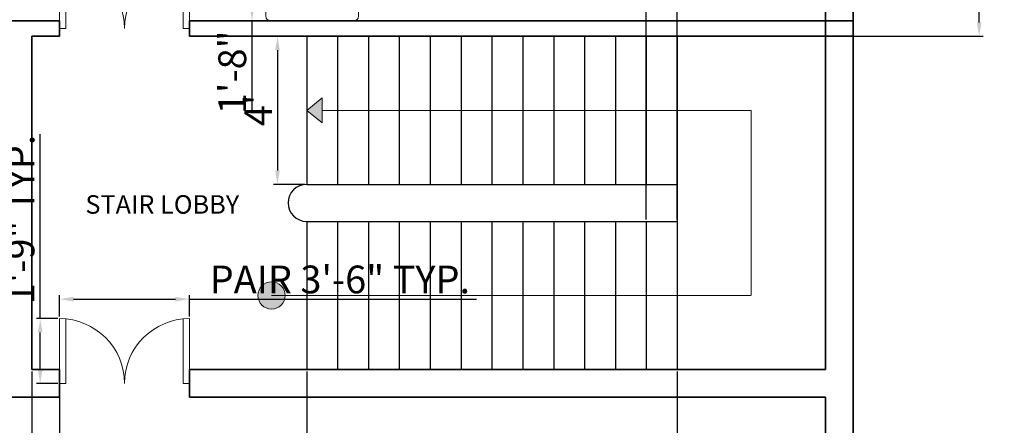
# Model space of a CAD drawing. Units: inches. Extents: x 1885 to 4781, y 1153 to 4395.
# Tile 4 of 7: x 2631 to 2950, y 1657 to 1789. Entities that reach past the tile are written whole.
import ezdxf

# ---------------------------------------------------------------- set-up
doc = ezdxf.new("R2010")
doc.units = ezdxf.units.IN
for name, color, linetype, lineweight in [('A-ANNO-DIMS', 5, 'Continuous', 18), ('A-ANNO-SYMB', 7, 'Continuous', 18), ('A-FLOR-STRS', 7, 'Continuous', 25), ('A-WALL', 7, 'Continuous', 35)]:
    doc.layers.add(name, color=color, linetype=linetype, lineweight=lineweight)
for name, color, linetype, lineweight, true_color in [('A-AREA-IDEN', 244, 'Continuous', 18, 0x991b1e), ('A-DOOR', 11, 'Continuous', 18, 0xf27172), ('A-FLOR-FIXT', 11, 'Continuous', 18, 0xf27172)]:
    doc.layers.add(name, color=color, linetype=linetype, lineweight=lineweight, true_color=true_color)
doc.styles.get("Standard").update_dxf_attribs({"font": 'arial.ttf'})
doc.dimstyles.new('ISO-25', dxfattribs={"dimtxt": 9, "dimasz": 4.5, "dimexe": 1.25, "dimexo": 0.625, "dimtad": 1, "dimdec": 0, "dimlunit": 3, "dimtxsty": 'Standard', "dimcen": 2.5, "dimadec": 0, "dimazin": 0, "dimtfac": 1, "dimtdec": 0, "dimtmove": 0, "dimatfit": 3, "dimfxl": 1, "dimarcsym": 0})

# ---------------------------------------------------------------- blocks, each defined once
blk = doc.blocks.new('Sink-single - 30 in top')
blk.add_line((-15, -3.999996), (15, -3.999996))
for points in [[(-13.5, 0), (13.5, 0)], [(-15, -18.499996), (-15, -1.5)], [(15, -1.5), (15, -18.499996)], [(-12.5, -5.499996), (12.5, -5.499996)], [(-13.5, -17.499996), (-13.5, -6.499996)], [(13.5, -6.499996), (13.5, -17.499996)], [(12.5, -18.499996), (-12.5, -18.499996)], [(13.5, -19.999996), (-13.5, -19.999996)]]:
    blk.add_lwpolyline(points)
for radius in [1, 0.5]:
    blk.add_circle((0, -11.999996), radius)
for centre, radius, start, end in [((-13.5, -1.5), 1.5, 90, 180), ((13.5, -1.5), 1.5, 0, 90), ((-12.5, -6.499996), 1, 90, 180), ((12.5, -6.499996), 1, 0, 90), ((-13.5, -18.499996), 1.5, 180, 270), ((-12.5, -17.499996), 1, 180, 270), ((12.5, -17.499996), 1, 270, 0), ((13.5, -18.499996), 1.5, 270, 0)]:
    blk.add_arc(centre, radius, start, end)
blk = doc.blocks.new('*D22')
at = {"layer": 'A-ANNO-DIMS', "color": 0, "lineweight": -2, "transparency": 16777216}
for p, q in [((2723.28, 1783.42), (2713.21, 1783.42)), ((2714.46, 1778.92), (2714.46, 1739.92)), ((2723.28, 1735.42), (2713.21, 1735.42))]:
    blk.add_line(p, q, dxfattribs=at)
at = {"layer": 'A-ANNO-DIMS', "color": 0, "transparency": 16777216}
for points in [[(2713.71, 1778.92), (2715.21, 1778.92), (2714.46, 1783.42)], [(2713.71, 1739.92), (2715.21, 1739.92), (2714.46, 1735.42)]]:
    blk.add_solid(points, dxfattribs=at)
at = {"layer": 'Defpoints', "color": 0, "transparency": 16777216}
for p in [(2723.91, 1783.42), (2714.46, 1735.42), (2723.91, 1735.42)]:
    blk.add_point(p, dxfattribs=at)
at = {"layer": 'A-ANNO-DIMS', "color": 0, "transparency": 16777216, "insert": (2709.34, 1759.42), "char_height": 9, "attachment_point": 5, "rotation": 90}
blk.add_mtext("4'", dxfattribs=at)
blk = doc.blocks.new('DOOR-PAIR-42IN')
for p, q in [((0, 21), (0, 0)), ((2, 21), (2, 0)), ((40, 21), (40, 0)), ((42, 21), (42, 0)), ((0, 0), (2, 0)), ((42, 0), (40, 0))]:
    blk.add_line(p, q)
for centre, start, end in [((0, 0), 0, 90), ((42, 0), 90, 180)]:
    blk.add_arc(centre, 21, start, end)
blk = doc.blocks.new('*D55')
at = {"layer": 'A-ANNO-DIMS', "color": 0, "lineweight": -2, "transparency": 16777216}
for p, q in [((2643.91, 1692.55), (2643.91, 1699.47)), ((2648.41, 1698.22), (2681.41, 1698.22)), ((2685.91, 1692.55), (2685.91, 1699.47)), ((2685.91, 1698.22), (2778.91, 1698.22))]:
    blk.add_line(p, q, dxfattribs=at)
at = {"layer": 'A-ANNO-DIMS', "color": 0, "transparency": 16777216}
for points in [[(2648.41, 1698.97), (2648.41, 1697.47), (2643.91, 1698.22)], [(2681.41, 1698.97), (2681.41, 1697.47), (2685.91, 1698.22)]]:
    blk.add_solid(points, dxfattribs=at)
at = {"layer": 'Defpoints', "color": 0, "transparency": 16777216}
for p in [(2685.91, 1698.22), (2643.91, 1691.92), (2685.91, 1691.92)]:
    blk.add_point(p, dxfattribs=at)
at = {"layer": 'A-ANNO-DIMS', "color": 0, "transparency": 16777216, "insert": (2734.66, 1703.44), "char_height": 9, "attachment_point": 5}
blk.add_mtext('PAIR 3\'-6" TYP.', dxfattribs=at)
blk = doc.blocks.new('*D56')
at = {"layer": 'A-ANNO-DIMS', "color": 0, "lineweight": -2, "transparency": 16777216}
for p, q in [((2637.61, 1691.92), (2637.61, 1751.68)), ((2643.28, 1691.92), (2636.36, 1691.92)), ((2637.61, 1675.42), (2637.61, 1687.42)), ((2643.28, 1670.92), (2636.36, 1670.92))]:
    blk.add_line(p, q, dxfattribs=at)
at = {"layer": 'A-ANNO-DIMS', "color": 0, "transparency": 16777216}
for points in [[(2636.86, 1687.42), (2638.36, 1687.42), (2637.61, 1691.92)], [(2636.86, 1675.42), (2638.36, 1675.42), (2637.61, 1670.92)]]:
    blk.add_solid(points, dxfattribs=at)
at = {"layer": 'Defpoints', "color": 0, "transparency": 16777216}
for p in [(2637.61, 1691.92), (2643.91, 1691.92), (2643.91, 1670.92)]:
    blk.add_point(p, dxfattribs=at)
at = {"layer": 'A-ANNO-DIMS', "color": 0, "transparency": 16777216, "insert": (2632.39, 1724.05), "char_height": 9, "attachment_point": 5, "rotation": 90}
blk.add_mtext('1\'-9" TYP.', dxfattribs=at)
blk = doc.blocks.new('*D72')
at = {"layer": 'A-ANNO-DIMS', "color": 0, "lineweight": -2, "transparency": 16777216}
for p, q in [((2710.07, 1808.42), (2704.94, 1808.42)), ((2706.19, 1803.92), (2706.19, 1792.92)), ((2710.07, 1788.42), (2704.94, 1788.42)), ((2706.19, 1788.42), (2706.19, 1759.59))]:
    blk.add_line(p, q, dxfattribs=at)
at = {"layer": 'A-ANNO-DIMS', "color": 0, "transparency": 16777216}
for points in [[(2705.44, 1803.92), (2706.94, 1803.92), (2706.19, 1808.42)], [(2705.44, 1792.92), (2706.94, 1792.92), (2706.19, 1788.42)]]:
    blk.add_solid(points, dxfattribs=at)
at = {"layer": 'Defpoints', "color": 0, "transparency": 16777216}
for p in [(2710.69, 1808.42), (2706.19, 1788.42), (2710.69, 1788.42)]:
    blk.add_point(p, dxfattribs=at)
at = {"layer": 'A-ANNO-DIMS', "color": 0, "transparency": 16777216, "insert": (2700.97, 1771.76), "char_height": 9, "attachment_point": 5, "rotation": 90}
blk.add_mtext('1\'-8"', dxfattribs=at)
blk = doc.blocks.new('*D75')
at = {"layer": 'A-ANNO-DIMS', "color": 0, "lineweight": -2, "transparency": 16777216}
for p, q in [((2723.91, 1674.8), (2723.91, 1447.37)), ((2843.91, 1674.8), (2843.91, 1447.37)), ((2728.41, 1448.62), (2839.41, 1448.62))]:
    blk.add_line(p, q, dxfattribs=at)
at = {"layer": 'A-ANNO-DIMS', "color": 0, "transparency": 16777216}
for points in [[(2728.41, 1449.37), (2728.41, 1447.87), (2723.91, 1448.62)], [(2839.41, 1449.37), (2839.41, 1447.87), (2843.91, 1448.62)]]:
    blk.add_solid(points, dxfattribs=at)
at = {"layer": 'Defpoints', "color": 0, "transparency": 16777216}
for p in [(2723.91, 1675.42), (2843.91, 1675.42), (2843.91, 1448.62)]:
    blk.add_point(p, dxfattribs=at)
at = {"layer": 'A-ANNO-DIMS', "color": 0, "transparency": 16777216, "insert": (2783.91, 1453.84), "char_height": 9, "attachment_point": 5}
blk.add_mtext('10\'-0"', dxfattribs=at)
blk = doc.blocks.new('*D89')
at = {"layer": 'A-ANNO-DIMS', "color": 0, "lineweight": -2, "transparency": 16777216}
for p, q in [((2941.71, 1827.92), (2941.71, 1878.56)), ((2892.53, 1827.92), (2942.96, 1827.92)), ((2941.71, 1787.92), (2941.71, 1823.42)), ((2892.53, 1783.42), (2942.96, 1783.42))]:
    blk.add_line(p, q, dxfattribs=at)
at = {"layer": 'A-ANNO-DIMS', "color": 0, "transparency": 16777216}
for points in [[(2940.96, 1823.42), (2942.46, 1823.42), (2941.71, 1827.92)], [(2940.96, 1787.92), (2942.46, 1787.92), (2941.71, 1783.42)]]:
    blk.add_solid(points, dxfattribs=at)
at = {"layer": 'Defpoints', "color": 0, "transparency": 16777216}
for p in [(2891.91, 1827.92), (2941.71, 1827.92), (2891.91, 1783.42)]:
    blk.add_point(p, dxfattribs=at)
at = {"layer": 'A-ANNO-DIMS', "color": 0, "transparency": 16777216, "insert": (2936.43, 1855.49), "char_height": 9, "attachment_point": 5, "rotation": 90}
blk.add_mtext('3\'-8 1/2"', dxfattribs=at)
blk = doc.blocks.new('*D91')
at = {"layer": 'A-ANNO-DIMS', "color": 0, "lineweight": -2, "transparency": 16777216}
for p, q in [((2634.91, 1674.8), (2634.91, 1447.37)), ((2643.91, 1674.8), (2643.91, 1447.37)), ((2630.41, 1448.62), (2625.91, 1448.62)), ((2634.91, 1448.62), (2643.91, 1448.62)), ((2648.41, 1448.62), (2678.08, 1448.62))]:
    blk.add_line(p, q, dxfattribs=at)
at = {"layer": 'A-ANNO-DIMS', "color": 0, "transparency": 16777216}
for points in [[(2630.41, 1449.37), (2630.41, 1447.87), (2634.91, 1448.62)], [(2648.41, 1449.37), (2648.41, 1447.87), (2643.91, 1448.62)]]:
    blk.add_solid(points, dxfattribs=at)
at = {"layer": 'Defpoints', "color": 0, "transparency": 16777216}
for p in [(2634.91, 1675.42), (2643.91, 1675.42), (2643.91, 1448.62)]:
    blk.add_point(p, dxfattribs=at)
at = {"layer": 'A-ANNO-DIMS', "color": 0, "transparency": 16777216, "insert": (2665.49, 1453.84), "char_height": 9, "attachment_point": 5}
blk.add_mtext('0\'-9"', dxfattribs=at)
blk = doc.blocks.new('*D92')
at = {"layer": 'A-ANNO-DIMS', "color": 0, "lineweight": -2, "transparency": 16777216}
for p, q in [((2833.91, 1724.05), (2833.91, 2264.47)), ((2843.91, 1724.05), (2843.91, 2264.47)), ((2829.41, 2263.22), (2824.91, 2263.22)), ((2833.91, 2263.22), (2843.91, 2263.22)), ((2848.41, 2263.22), (2885.07, 2263.22))]:
    blk.add_line(p, q, dxfattribs=at)
at = {"layer": 'A-ANNO-DIMS', "color": 0, "transparency": 16777216}
for points in [[(2829.41, 2263.97), (2829.41, 2262.47), (2833.91, 2263.22)], [(2848.41, 2263.97), (2848.41, 2262.47), (2843.91, 2263.22)]]:
    blk.add_solid(points, dxfattribs=at)
at = {"layer": 'Defpoints', "color": 0, "transparency": 16777216}
for p in [(2843.91, 2263.22), (2833.91, 1723.42), (2843.91, 1723.42)]:
    blk.add_point(p, dxfattribs=at)
at = {"layer": 'A-ANNO-DIMS', "color": 0, "transparency": 16777216, "insert": (2868.99, 2268.44), "char_height": 9, "attachment_point": 5}
blk.add_mtext('0\'-10"', dxfattribs=at)

msp = doc.modelspace()

# ---------------------------------------------------------------- hatches: boundary and pattern name
at = {"layer": 'A-ANNO-SYMB'}
h = msp.add_hatch(color=256, dxfattribs=at)
h.dxf.hatch_style = 1
h.paths.add_polyline_path([(2728.98, 1763.47), (2723.91, 1759.42), (2728.98, 1755.37)])
h = msp.add_hatch(color=256, dxfattribs=at)
h.dxf.hatch_style = 1
h.paths.add_polyline_path([(2708.14, 1699.42, 1), (2716.97, 1699.42, 1)])

# ---------------------------------------------------------------- linework, layer by layer
for p, q in [((2723.91, 1759.42), (2728.98, 1763.47)), ((2728.98, 1763.47), (2728.98, 1755.37)), ((2723.91, 1759.42), (2728.98, 1755.37)), ((2867.91, 1759.42), (2728.98, 1759.42)), ((2867.91, 1759.42), (2867.91, 1699.42)), ((2723.91, 1699.42), (2712.55, 1699.42)), ((2723.91, 1699.42), (2867.61, 1699.42))]:
    msp.add_line(p, q, dxfattribs=at)
msp.add_circle((2712.55, 1699.42), 4.41, dxfattribs=at)
at = {"layer": 'A-FLOR-STRS'}
for p, q in [((2723.91, 1783.42), (2723.91, 1735.42)), ((2733.91, 1783.42), (2733.91, 1735.42)), ((2743.91, 1783.42), (2743.91, 1735.42)), ((2753.91, 1783.42), (2753.91, 1735.42)), ((2763.91, 1783.42), (2763.91, 1735.42)), ((2773.91, 1783.42), (2773.91, 1735.42)), ((2783.91, 1783.42), (2783.91, 1735.42)), ((2793.91, 1783.42), (2793.91, 1735.42)), ((2803.91, 1783.42), (2803.91, 1735.42)), ((2813.91, 1783.42), (2813.91, 1735.42)), ((2823.91, 1783.42), (2823.91, 1735.42)), ((2833.91, 1783.42), (2833.91, 1735.42)), ((2843.91, 1783.42), (2843.91, 1735.42)), ((2891.91, 1783.42), (2891.91, 1675.42)), ((2723.91, 1735.42), (2843.91, 1735.42)), ((2843.91, 1735.42), (2843.91, 1723.42)), ((2723.91, 1723.42), (2843.91, 1723.42)), ((2723.91, 1723.42), (2723.91, 1675.42)), ((2733.91, 1723.42), (2733.91, 1675.42)), ((2743.91, 1723.42), (2743.91, 1675.42)), ((2753.91, 1723.42), (2753.91, 1675.42)), ((2763.91, 1723.42), (2763.91, 1675.42)), ((2773.91, 1723.42), (2773.91, 1675.42)), ((2783.91, 1723.42), (2783.91, 1675.42)), ((2793.91, 1723.42), (2793.91, 1675.42)), ((2803.91, 1723.42), (2803.91, 1675.42)), ((2813.91, 1723.42), (2813.91, 1675.42)), ((2823.91, 1723.42), (2823.91, 1675.42)), ((2833.91, 1723.42), (2833.91, 1675.42)), ((2843.91, 1723.42), (2843.91, 1675.42))]:
    msp.add_line(p, q, dxfattribs=at)
msp.add_arc((2723.91, 1729.42), 6, 90, 270, dxfattribs=at)
at = {"layer": 'A-WALL'}
for p, q in [((2900.91, 2222.42), (2900.91, 1489.42)), ((2891.91, 2028.42), (2891.91, 1675.42)), ((2623.91, 1788.42), (2643.91, 1788.42)), ((2643.91, 1788.42), (2643.91, 1783.42)), ((2643.91, 1788.42), (2643.91, 1783.42)), ((2685.91, 1788.42), (2685.91, 1783.42)), ((2685.91, 1788.42), (2900.91, 1788.42)), ((2685.91, 1788.42), (2685.91, 1783.42)), ((2634.91, 1783.42), (2634.91, 1675.42)), ((2634.91, 1783.42), (2643.91, 1783.42)), ((2685.91, 1783.42), (2900.91, 1783.42)), ((2634.91, 1675.42), (2643.91, 1675.42)), ((2643.91, 1675.42), (2643.91, 1666.42)), ((2685.91, 1675.42), (2685.91, 1666.42)), ((2685.91, 1675.42), (2891.91, 1675.42)), ((2560.91, 1666.42), (2643.91, 1666.42)), ((2685.91, 1666.42), (2891.91, 1666.42)), ((2891.91, 1666.42), (2891.91, 1498.42))]:
    msp.add_line(p, q, dxfattribs=at)

# ---------------------------------------------------------------- block references
at = {"layer": 'A-DOOR'}
for p in [(2643.91, 1785.92), (2643.91, 1670.92)]:
    msp.add_blockref('DOOR-PAIR-42IN', p, dxfattribs=at)
at = {"layer": 'A-FLOR-FIXT', "rotation": 180}
msp.add_blockref('Sink-single - 30 in top', (2725.69, 1788.42), dxfattribs=at)

# ---------------------------------------------------------------- texts
at = {"layer": 'A-AREA-IDEN'}
msp.add_text('STAIR LOBBY', height=6, dxfattribs=at).set_placement((2652.25, 1725.92))

# ---------------------------------------------------------------- dimensions: what is measured, and where the dimension line sits
at = {"layer": 'A-ANNO-DIMS'}
for base, p1, p2, picture, middle in [((2843.91, 2263.22), (2833.91, 1723.42), (2843.91, 1723.42), '*D92', (2868.99, 2268.44)), ((2643.91, 1448.62), (2634.91, 1675.42), (2643.91, 1675.42), '*D91', (2665.49, 1453.84)), ((2843.91, 1448.62), (2723.91, 1675.42), (2843.91, 1675.42), '*D75', (2783.91, 1453.84))]:
    dim = msp.add_linear_dim(base=base, p1=p1, p2=p2, dimstyle='ISO-25', override={"dimdec": 1, "dimlfac": 1, "dimrnd": 0, "dimzin": 1, "dimdsep": 46, "dimlunit": 4, "dimfrac": 2}, dxfattribs=at)
    dim.commit()
    dim.dimension.update_dxf_attribs({"geometry": picture, "text_midpoint": middle})
for base, p1, p2, angle, override, picture, middle in [((2941.71, 1827.92), (2891.91, 1783.42), (2891.91, 1827.92), 90, {"dimdec": 1, "dimlfac": 1, "dimrnd": 0, "dimzin": 1, "dimdsep": 46, "dimlunit": 4, "dimfrac": 2}, '*D89', (2936.43, 1855.49)), ((2706.19, 1788.42), (2710.69, 1808.42), (2710.69, 1788.42), 270, {"dimdec": 1, "dimlfac": 1, "dimrnd": 0, "dimzin": 1, "dimdsep": 46, "dimlunit": 4, "dimfrac": 2}, '*D72', (2700.97, 1771.76)), ((2714.46, 1735.42), (2723.91, 1783.42), (2723.91, 1735.42), 90, {"dimclrd": 0, "dimclre": 0, "dimclrt": 0}, '*D22', (2709.34, 1759.42))]:
    dim = msp.add_linear_dim(base=base, p1=p1, p2=p2, angle=angle, dimstyle='ISO-25', override=override, dxfattribs=at)
    dim.commit()
    dim.dimension.update_dxf_attribs({"geometry": picture, "text_midpoint": middle})
dim = msp.add_linear_dim(base=(2637.61, 1691.92), p1=(2643.91, 1670.92), p2=(2643.91, 1691.92), angle=90, text='<> TYP.', dimstyle='ISO-25', override={"dimdec": 1, "dimlfac": 1, "dimrnd": 0, "dimzin": 1, "dimdsep": 46, "dimlunit": 4, "dimfrac": 2}, dxfattribs=at)
dim.commit()
dim.dimension.update_dxf_attribs({"geometry": '*D56', "text_midpoint": (2632.39, 1724.05)})
dim = msp.add_linear_dim(base=(2685.91, 1698.22), p1=(2643.91, 1691.92), p2=(2685.91, 1691.92), text='PAIR <> TYP.', dimstyle='ISO-25', override={"dimdec": 1, "dimlfac": 1, "dimrnd": 0, "dimzin": 1, "dimdsep": 46, "dimlunit": 4, "dimfrac": 2}, dxfattribs=at)
dim.commit()
dim.dimension.update_dxf_attribs({"geometry": '*D55', "text_midpoint": (2734.66, 1703.44)})

doc.saveas('drawing.dxf')
